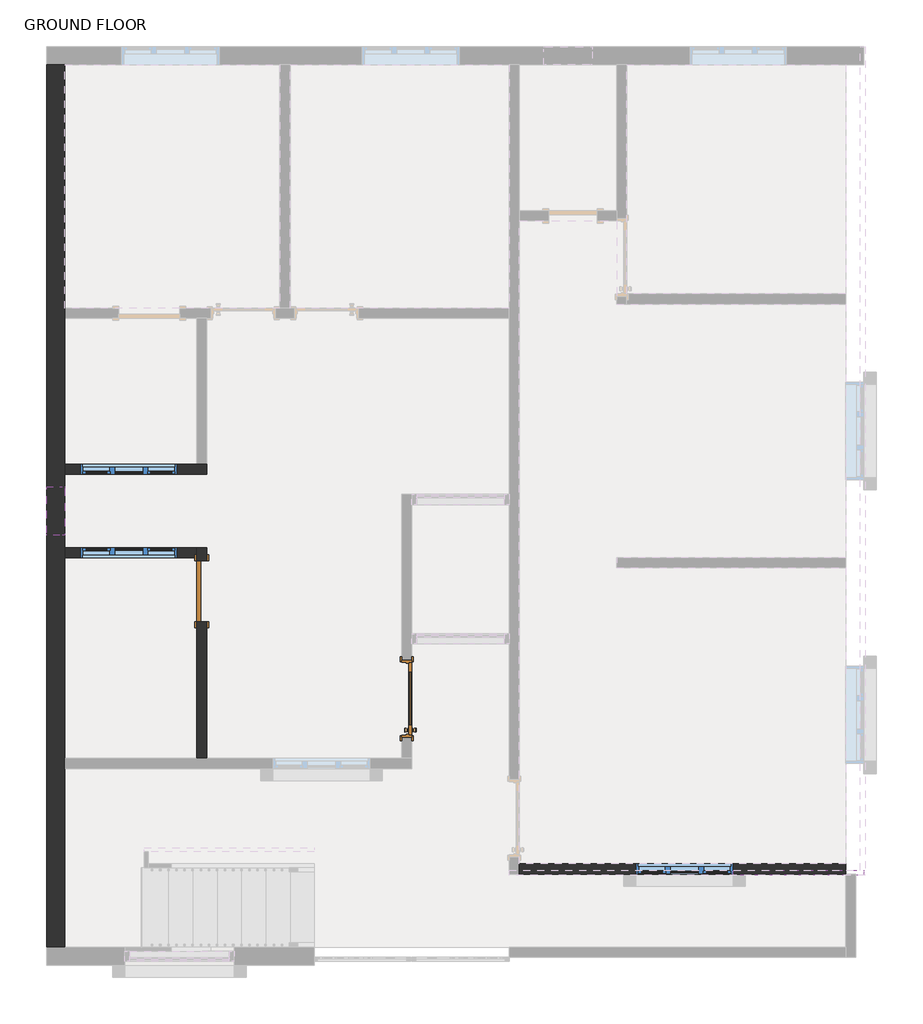
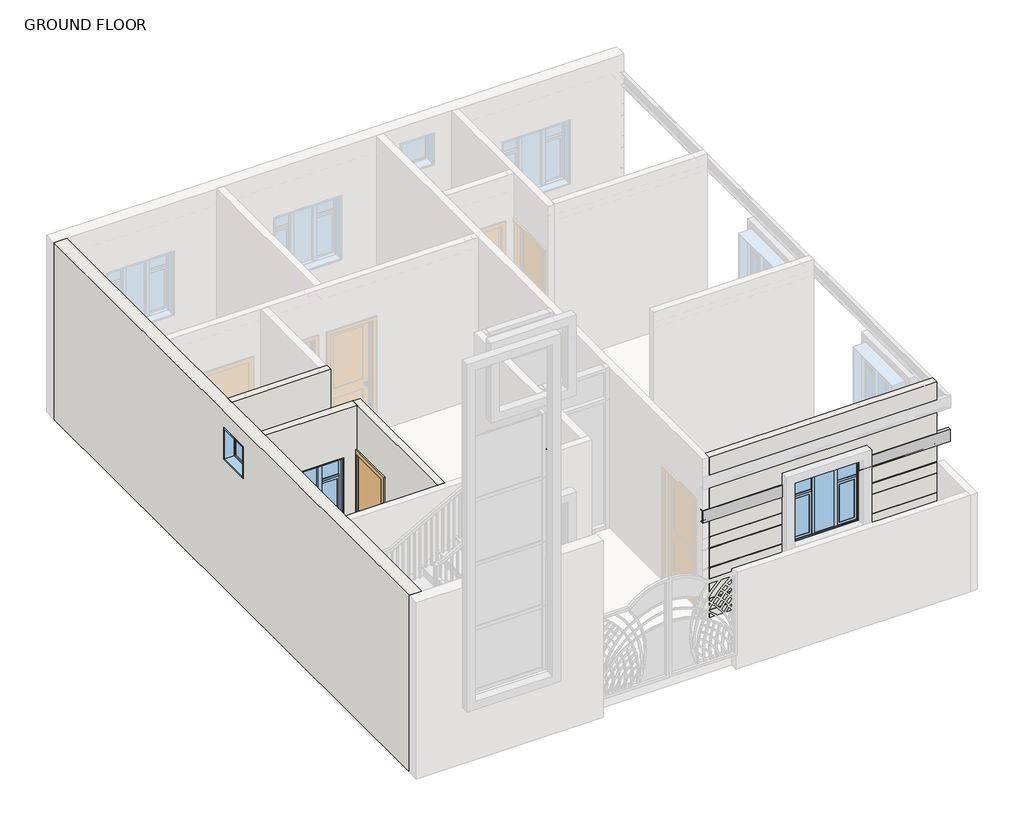
# One storey, part 2 of 7: 5 walls, 4 windows, 2 doors, 1 proxy.
"""IFC4 building model written with IfcOpenShell, lengths in millimetres."""

from ifc_helpers import new_model, si_unit, point, frame, frame_2d, origin, place, context, project, spatial, polyline, circle_curve, trimmed, segment, composite_curve, outline, extrude, faceted_brep, transform, mapped, element, save
from ifc_brep_helpers import plane_surface, cylinder_surface, revolved_surface, advanced_brep
from components import door_2e56f206, single_flush_bathroom_flush_door_4d6c7550, fixed_opening_window_2_x_2_e119d648, window_casement_triple_side_transom_window_4_x_4_9406f89d

model = new_model("IFC4")

# Units and contexts
model_context = context("Model", 3, world=origin())
ifc_project = project(units=[si_unit("LENGTHUNIT", "METRE", prefix="MILLI")], contexts=[model_context])

# Site, building, storey
site = spatial("IfcSite", under=ifc_project)
building = spatial("IfcBuilding", under=site)
storey = spatial("IfcBuildingStorey", under=building, Name="GROUND FLOOR", Elevation=304.8)

# Proxy
placement = place(None, origin())
element("IfcBuildingElementProxy", 1, Name="Reveal", ObjectType="Reveal", at=placement, inside=storey, context=model_context, shape_type="SweptSolid", body=[
    extrude(outline(composite_curve([segment(polyline([(-1857.2343863, 2374.9), (-1793.9883863, 2374.9), (-1793.9883863, 2373.5203242)]), True, "CONTINUOUS"), segment(trimmed(circle_curve(frame_2d((-1799.2334863, 2373.5203242)), 5.2451), [point((-1793.9883863, 2373.5203242))], [point((-1798.3711955, 2368.3465897))], False, "CARTESIAN"), True, "CONTINUOUS"), segment(polyline([(-1798.3711955, 2368.3465897), (-1821.9918863, 2364.4098), (-1841.2297679, 2361.20348)]), True, "CONTINUOUS"), segment(trimmed(circle_curve(frame_2d((-1839.5051863, 2350.856011)), 10.4902), [point((-1841.2297679, 2361.20348))], [point((-1849.9953863, 2350.856011))], True, "CARTESIAN"), True, "CONTINUOUS"), segment(polyline([(-1849.9953863, 2350.856011), (-1849.9953863, 2170.343989)]), True, "CONTINUOUS"), segment(trimmed(circle_curve(frame_2d((-1839.5051863, 2170.343989)), 10.4902), [point((-1849.9953863, 2170.343989))], [point((-1841.2297679, 2159.99652))], True, "CARTESIAN"), True, "CONTINUOUS"), segment(polyline([(-1841.2297679, 2159.99652), (-1821.9918863, 2156.7902), (-1798.3711955, 2152.8534103)]), True, "CONTINUOUS"), segment(trimmed(circle_curve(frame_2d((-1799.2334863, 2147.6796758)), 5.2451), [point((-1798.3711955, 2152.8534103))], [point((-1793.9883863, 2147.6796758))], False, "CARTESIAN"), True, "CONTINUOUS"), segment(polyline([(-1793.9883863, 2147.6796758), (-1793.9883863, 2146.3), (-1857.2343863, 2146.3), (-1857.2343863, 2374.9)]), True, "CONTINUOUS")], self_intersect=False)), frame((-6391.4023867, 0.0, 0.0), z_axis=(1.0, 0.0, 0.0), x_axis=(0.0, 1.0, 0.0)), (0.0, 0.0, 1.0), 1638.3),
    extrude(outline(composite_curve([segment(polyline([(-1857.2343863, 2374.9), (-1793.9883863, 2374.9), (-1793.9883863, 2373.5203242)]), True, "CONTINUOUS"), segment(trimmed(circle_curve(frame_2d((-1799.2334863, 2373.5203242)), 5.2451), [point((-1793.9883863, 2373.5203242))], [point((-1798.3711955, 2368.3465897))], False, "CARTESIAN"), True, "CONTINUOUS"), segment(polyline([(-1798.3711955, 2368.3465897), (-1821.9918863, 2364.4098), (-1841.2297679, 2361.20348)]), True, "CONTINUOUS"), segment(trimmed(circle_curve(frame_2d((-1839.5051863, 2350.856011)), 10.4902), [point((-1841.2297679, 2361.20348))], [point((-1849.9953863, 2350.856011))], True, "CARTESIAN"), True, "CONTINUOUS"), segment(polyline([(-1849.9953863, 2350.856011), (-1849.9953863, 2170.343989)]), True, "CONTINUOUS"), segment(trimmed(circle_curve(frame_2d((-1839.5051863, 2170.343989)), 10.4902), [point((-1849.9953863, 2170.343989))], [point((-1841.2297679, 2159.99652))], True, "CARTESIAN"), True, "CONTINUOUS"), segment(polyline([(-1841.2297679, 2159.99652), (-1821.9918863, 2156.7902), (-1798.3711955, 2152.8534103)]), True, "CONTINUOUS"), segment(trimmed(circle_curve(frame_2d((-1799.2334863, 2147.6796758)), 5.2451), [point((-1798.3711955, 2152.8534103))], [point((-1793.9883863, 2147.6796758))], False, "CARTESIAN"), True, "CONTINUOUS"), segment(polyline([(-1793.9883863, 2147.6796758), (-1793.9883863, 2146.3), (-1857.2343863, 2146.3), (-1857.2343863, 2374.9)]), True, "CONTINUOUS")], self_intersect=False)), frame((-9198.1023867, 0.0, 0.0), z_axis=(1.0, 0.0, 0.0), x_axis=(0.0, 1.0, 0.0)), (0.0, 0.0, 1.0), 1587.5),
])

# Doors
door_shape = door_2e56f206(model_context)
element("IfcDoor", 2, ObjectType="Door-Interior-Single-2_Panel-Wood : 36\" x 84\"", at=placement, inside=storey, context=model_context, shape_type="MappedRepresentation", body=[
    mapped(door_shape, transform((-10477.6273867, 354.7500137, 304.8), x_axis=(0.0, 1.0, 0.0), y_axis=(-1.0, 0.0, 0.0), z_axis=(0.0, 0.0, 1.0))),
])
single_flush_bathroom_flush_door_shape = single_flush_bathroom_flush_door_4d6c7550(model_context)
element("IfcDoor", 3, ObjectType="Single-Flush : BATHROOM FLUSH DOOR", at=placement, inside=storey, context=model_context, shape_type="MappedRepresentation", body=[
    mapped(single_flush_bathroom_flush_door_shape, transform((-13046.2023867, 1700.5265627, 304.8), x_axis=(0.0, 1.0, 0.0), y_axis=(-1.0, 0.0, 0.0), z_axis=(0.0, 0.0, 1.0))),
])

# Walls
element("IfcWall", 4, at=placement, inside=storey, context=model_context, shape_type="Brep", body=[
    faceted_brep([(-14760.7023867, -2756.7499863, 0.0), (-14760.7023867, 8292.2500137, 0.0), (-14760.7023867, 8292.2500137, 3352.8), (-14760.7023867, 5244.2500137, 3352.8), (-14760.7023867, 5117.2500137, 3352.8), (-14760.7023867, 3288.4500137, 3352.8), (-14760.7023867, 3161.4500137, 3352.8), (-14760.7023867, 2246.6265627, 3352.8), (-14760.7023867, 2119.6265627, 3352.8), (-14760.7023867, -394.5499863, 3352.8), (-14760.7023867, -521.5499863, 3352.8), (-14760.7023867, -2756.7499863, 3352.8), (-14760.7023867, 2399.2382882, 2438.4), (-14760.7023867, 2399.2382882, 3048.0), (-14760.7023867, 3008.8382882, 3048.0), (-14760.7023867, 3008.8382882, 2438.4), (-14989.3023867, 8292.2500137, 0.0), (-14989.3023867, -2756.7499863, 0.0), (-14989.3023867, -2756.7499863, 3352.8), (-14989.3023867, 8292.2500137, 3352.8), (-14989.3023867, 2399.2382882, 3048.0), (-14989.3023867, 2399.2382882, 2438.4), (-14989.3023867, 3008.8382882, 2438.4), (-14989.3023867, 3008.8382882, 3048.0)], [[[0, 1, 2, 3, 4, 5, 6, 7, 8, 9, 10, 11], [12, 13, 14, 15]], [[16, 17, 18, 19], [20, 21, 22, 23]], [[1, 0, 17, 16]], [[11, 10, 9, 8, 7, 6, 5, 4, 3, 2, 19, 18]], [[0, 11, 18, 17]], [[2, 1, 16, 19]], [[20, 13, 12, 21]], [[21, 12, 15, 22]], [[22, 15, 14, 23]], [[13, 20, 23, 14]]]),
])
element("IfcWall", 5, ObjectType="INNER WALL 5\"", at=placement, inside=storey, context=model_context, shape_type="AdvancedBrep", body=[
    advanced_brep(
    [(-9071.1023867, -1842.3499863, 0.0), (-4981.7023867, -1842.3499863, 0.0), (-4981.7023867, -1842.3499863, 444.5), (-9071.1023867, -1842.3499863, 444.5), (-9071.1023867, -1842.3499863, 304.8), (-4981.7023867, -1842.3499863, 3352.8), (-9071.1023867, -1842.3499863, 3352.8), (-9071.1023867, -1842.3499863, 3009.9), (-4981.7023867, -1842.3499863, 3009.9), (-6391.4023867, -1842.3499863, 1219.2), (-7610.6023867, -1842.3499863, 1219.2), (-7610.6023867, -1842.3499863, 1243.35311), (-9071.1023867, -1842.3499863, 1243.35311), (-9071.1023867, -1842.3499863, 1042.64689), (-4981.7023867, -1842.3499863, 1042.64689), (-4981.7023867, -1842.3499863, 1243.35311), (-6391.4023867, -1842.3499863, 1243.35311), (-7610.6023867, -1842.3499863, 2438.4), (-6391.4023867, -1842.3499863, 2438.4), (-6391.4023867, -1842.3499863, 2374.9), (-4981.7023867, -1842.3499863, 2374.9), (-4981.7023867, -1842.3499863, 2781.3), (-9071.1023867, -1842.3499863, 2781.3), (-9071.1023867, -1842.3499863, 2374.9), (-7610.6023867, -1842.3499863, 2374.9), (-4981.7023867, -1842.3499863, 2795.24689), (-4981.7023867, -1842.3499863, 2995.95311), (-9071.1023867, -1842.3499863, 2995.95311), (-9071.1023867, -1842.3499863, 2795.24689), (-9071.1023867, -1842.3499863, 673.1), (-4981.7023867, -1842.3499863, 673.1), (-4981.7023867, -1842.3499863, 1028.7), (-9071.1023867, -1842.3499863, 1028.7), (-4981.7023867, -1842.3499863, 659.15311), (-9071.1023867, -1842.3499863, 659.15311), (-9071.1023867, -1842.3499863, 458.44689), (-4981.7023867, -1842.3499863, 458.44689), (-9071.1023867, -1842.3499863, 1257.3), (-7610.6023867, -1842.3499863, 1257.3), (-7610.6023867, -1842.3499863, 1612.9), (-9071.1023867, -1842.3499863, 1612.9), (-6391.4023867, -1842.3499863, 1257.3), (-4981.7023867, -1842.3499863, 1257.3), (-4981.7023867, -1842.3499863, 1612.9), (-6391.4023867, -1842.3499863, 1612.9), (-6391.4023867, -1842.3499863, 1841.5), (-4981.7023867, -1842.3499863, 1841.5), (-4981.7023867, -1842.3499863, 2146.3), (-6391.4023867, -1842.3499863, 2146.3), (-4981.7023867, -1842.3499863, 1827.55311), (-6391.4023867, -1842.3499863, 1827.55311), (-6391.4023867, -1842.3499863, 1626.84689), (-4981.7023867, -1842.3499863, 1626.84689), (-9071.1023867, -1842.3499863, 1841.5), (-7610.6023867, -1842.3499863, 1841.5), (-7610.6023867, -1842.3499863, 2146.3), (-9071.1023867, -1842.3499863, 2146.3), (-7610.6023867, -1842.3499863, 1827.55311), (-9071.1023867, -1842.3499863, 1827.55311), (-9071.1023867, -1842.3499863, 1626.84689), (-7610.6023867, -1842.3499863, 1626.84689), (-6391.4023867, -1842.3499863, 2360.95311), (-6391.4023867, -1842.3499863, 2160.24689), (-4981.7023867, -1842.3499863, 2160.24689), (-4981.7023867, -1842.3499863, 2360.95311), (-9071.1023867, -1842.3499863, 2360.95311), (-9071.1023867, -1842.3499863, 2160.24689), (-7610.6023867, -1842.3499863, 2160.24689), (-7610.6023867, -1842.3499863, 2360.95311), (-4981.7023867, -1715.3499863, 0.0), (-9071.1023867, -1715.3499863, 0.0), (-9071.1023867, -1715.3499863, 3352.8), (-4981.7023867, -1715.3499863, 3352.8), (-7610.6023867, -1715.3499863, 2438.4), (-7610.6023867, -1715.3499863, 1219.2), (-6391.4023867, -1715.3499863, 1219.2), (-6391.4023867, -1715.3499863, 2438.4), (-9071.1023867, -1793.9883863, 444.5), (-9071.1023867, -1793.9883863, 445.8796758), (-9071.1023867, -1798.3711955, 451.0534103), (-9071.1023867, -1841.2297679, 458.19652), (-9071.1023867, -1841.2297679, 659.40348), (-9071.1023867, -1798.3711955, 666.5465897), (-9071.1023867, -1793.9883863, 671.7203242), (-9071.1023867, -1793.9883863, 673.1), (-9071.1023867, -1793.9883863, 1028.7), (-9071.1023867, -1793.9883863, 1030.0796758), (-9071.1023867, -1798.3711955, 1035.2534103), (-9071.1023867, -1841.2297679, 1042.39652), (-9071.1023867, -1841.2297679, 1243.60348), (-9071.1023867, -1798.3711955, 1250.7465897), (-9071.1023867, -1793.9883863, 1255.9203242), (-9071.1023867, -1793.9883863, 1257.3), (-9071.1023867, -1793.9883863, 1612.9), (-9071.1023867, -1793.9883863, 1614.2796758), (-9071.1023867, -1798.3711955, 1619.4534103), (-9071.1023867, -1841.2297679, 1626.59652), (-9071.1023867, -1841.2297679, 1827.80348), (-9071.1023867, -1798.3711955, 1834.9465897), (-9071.1023867, -1793.9883863, 1840.1203242), (-9071.1023867, -1793.9883863, 1841.5), (-9071.1023867, -1793.9883863, 2146.3), (-9071.1023867, -1793.9883863, 2147.6796758), (-9071.1023867, -1798.3711955, 2152.8534103), (-9071.1023867, -1841.2297679, 2159.99652), (-9071.1023867, -1841.2297679, 2361.20348), (-9071.1023867, -1798.3711955, 2368.3465897), (-9071.1023867, -1793.9883863, 2373.5203242), (-9071.1023867, -1793.9883863, 2374.9), (-9071.1023867, -1793.9883863, 2781.3), (-9071.1023867, -1793.9883863, 2782.6796758), (-9071.1023867, -1798.3711955, 2787.8534103), (-9071.1023867, -1841.2297679, 2794.99652), (-9071.1023867, -1841.2297679, 2996.20348), (-9071.1023867, -1798.3711955, 3003.3465897), (-9071.1023867, -1793.9883863, 3008.5203242), (-9071.1023867, -1793.9883863, 3009.9), (-7610.6023867, -1793.9883863, 2374.9), (-7610.6023867, -1793.9883863, 2373.5203242), (-7610.6023867, -1798.3711955, 2368.3465897), (-7610.6023867, -1841.2297679, 2361.20348), (-7610.6023867, -1841.2297679, 2159.99652), (-7610.6023867, -1798.3711955, 2152.8534103), (-7610.6023867, -1793.9883863, 2147.6796758), (-7610.6023867, -1793.9883863, 2146.3), (-7610.6023867, -1793.9883863, 1841.5), (-7610.6023867, -1793.9883863, 1840.1203242), (-7610.6023867, -1798.3711955, 1834.9465897), (-7610.6023867, -1841.2297679, 1827.80348), (-7610.6023867, -1841.2297679, 1626.59652), (-7610.6023867, -1798.3711955, 1619.4534103), (-7610.6023867, -1793.9883863, 1614.2796758), (-7610.6023867, -1793.9883863, 1612.9), (-7610.6023867, -1793.9883863, 1257.3), (-7610.6023867, -1793.9883863, 1255.9203242), (-7610.6023867, -1798.3711955, 1250.7465897), (-7610.6023867, -1841.2297679, 1243.60348), (-6391.4023867, -1841.2297679, 1243.60348), (-6391.4023867, -1798.3711955, 1250.7465897), (-6391.4023867, -1793.9883863, 1255.9203242), (-6391.4023867, -1793.9883863, 1257.3), (-6391.4023867, -1793.9883863, 1612.9), (-6391.4023867, -1793.9883863, 1614.2796758), (-6391.4023867, -1798.3711955, 1619.4534103), (-6391.4023867, -1841.2297679, 1626.59652), (-6391.4023867, -1841.2297679, 1827.80348), (-6391.4023867, -1798.3711955, 1834.9465897), (-6391.4023867, -1793.9883863, 1840.1203242), (-6391.4023867, -1793.9883863, 1841.5), (-6391.4023867, -1793.9883863, 2146.3), (-6391.4023867, -1793.9883863, 2147.6796758), (-6391.4023867, -1798.3711955, 2152.8534103), (-6391.4023867, -1841.2297679, 2159.99652), (-6391.4023867, -1841.2297679, 2361.20348), (-6391.4023867, -1798.3711955, 2368.3465897), (-6391.4023867, -1793.9883863, 2373.5203242), (-6391.4023867, -1793.9883863, 2374.9), (-4981.7023867, -1793.9883863, 3009.9), (-4981.7023867, -1793.9883863, 3008.5203242), (-4981.7023867, -1798.3711955, 3003.3465897), (-4981.7023867, -1841.2297679, 2996.20348), (-4981.7023867, -1841.2297679, 2794.99652), (-4981.7023867, -1798.3711955, 2787.8534103), (-4981.7023867, -1793.9883863, 2782.6796758), (-4981.7023867, -1793.9883863, 2781.3), (-4981.7023867, -1793.9883863, 2374.9), (-4981.7023867, -1793.9883863, 2373.5203242), (-4981.7023867, -1798.3711955, 2368.3465897), (-4981.7023867, -1841.2297679, 2361.20348), (-4981.7023867, -1841.2297679, 2159.99652), (-4981.7023867, -1798.3711955, 2152.8534103), (-4981.7023867, -1793.9883863, 2147.6796758), (-4981.7023867, -1793.9883863, 2146.3), (-4981.7023867, -1793.9883863, 1841.5), (-4981.7023867, -1793.9883863, 1840.1203242), (-4981.7023867, -1798.3711955, 1834.9465897), (-4981.7023867, -1841.2297679, 1827.80348), (-4981.7023867, -1841.2297679, 1626.59652), (-4981.7023867, -1798.3711955, 1619.4534103), (-4981.7023867, -1793.9883863, 1614.2796758), (-4981.7023867, -1793.9883863, 1612.9), (-4981.7023867, -1793.9883863, 1257.3), (-4981.7023867, -1793.9883863, 1255.9203242), (-4981.7023867, -1798.3711955, 1250.7465897), (-4981.7023867, -1841.2297679, 1243.60348), (-4981.7023867, -1841.2297679, 1042.39652), (-4981.7023867, -1798.3711955, 1035.2534103), (-4981.7023867, -1793.9883863, 1030.0796758), (-4981.7023867, -1793.9883863, 1028.7), (-4981.7023867, -1793.9883863, 673.1), (-4981.7023867, -1793.9883863, 671.7203242), (-4981.7023867, -1798.3711955, 666.5465897), (-4981.7023867, -1841.2297679, 659.40348), (-4981.7023867, -1841.2297679, 458.19652), (-4981.7023867, -1798.3711955, 451.0534103), (-4981.7023867, -1793.9883863, 445.8796758), (-4981.7023867, -1793.9883863, 444.5)],
    [
        (0, 1),
        (1, 2),
        (2, 3),
        (3, 4),
        (4, 0),
        (5, 6),
        (6, 7),
        (7, 8),
        (8, 5),
        (9, 10),
        (10, 11),
        (11, 12),
        (12, 13),
        (13, 14),
        (14, 15),
        (15, 16),
        (16, 9),
        (17, 18),
        (18, 19),
        (19, 20),
        (20, 21),
        (21, 22),
        (22, 23),
        (23, 24),
        (24, 17),
        (25, 26),
        (26, 27),
        (27, 28),
        (28, 25),
        (29, 30),
        (30, 31),
        (31, 32),
        (32, 29),
        (33, 34),
        (34, 35),
        (35, 36),
        (36, 33),
        (37, 38),
        (38, 39),
        (39, 40),
        (40, 37),
        (41, 42),
        (42, 43),
        (43, 44),
        (44, 41),
        (45, 46),
        (46, 47),
        (47, 48),
        (48, 45),
        (49, 50),
        (50, 51),
        (51, 52),
        (52, 49),
        (53, 54),
        (54, 55),
        (55, 56),
        (56, 53),
        (57, 58),
        (58, 59),
        (59, 60),
        (60, 57),
        (61, 62),
        (62, 63),
        (63, 64),
        (64, 61),
        (65, 66),
        (66, 67),
        (67, 68),
        (68, 65),
        (69, 70),
        (70, 71),
        (71, 72),
        (72, 69),
        (73, 74),
        (74, 75),
        (75, 76),
        (76, 73),
        (0, 70),
        (69, 1),
        (5, 72),
        (71, 6),
        (3, 77),
        (77, 78),
        (78, 79, circle_curve(frame((-9071.1023867, -1799.2334863, 445.8796758), z_axis=(1.0, 0.0, 0.0), x_axis=(0.0, 1.0, 0.0)), 5.2451)),
        (79, 80),
        (80, 35, circle_curve(frame((-9071.1023867, -1839.5051863, 468.543989), z_axis=(-1.0, 0.0, 0.0), x_axis=(0.0, 1.0, 0.0)), 10.4902)),
        (34, 81, circle_curve(frame((-9071.1023867, -1839.5051863, 649.056011), z_axis=(-1.0, 0.0, 0.0), x_axis=(0.0, 1.0, 0.0)), 10.4902)),
        (81, 82),
        (82, 83, circle_curve(frame((-9071.1023867, -1799.2334863, 671.7203242), z_axis=(1.0, 0.0, 0.0), x_axis=(0.0, 1.0, 0.0)), 5.2451)),
        (83, 84),
        (84, 29),
        (32, 85),
        (85, 86),
        (86, 87, circle_curve(frame((-9071.1023867, -1799.2334863, 1030.0796758), z_axis=(1.0, 0.0, 0.0), x_axis=(0.0, 1.0, 0.0)), 5.2451)),
        (87, 88),
        (88, 13, circle_curve(frame((-9071.1023867, -1839.5051863, 1052.743989), z_axis=(-1.0, 0.0, 0.0), x_axis=(0.0, 1.0, 0.0)), 10.4902)),
        (12, 89, circle_curve(frame((-9071.1023867, -1839.5051863, 1233.256011), z_axis=(-1.0, 0.0, 0.0), x_axis=(0.0, 1.0, 0.0)), 10.4902)),
        (89, 90),
        (90, 91, circle_curve(frame((-9071.1023867, -1799.2334863, 1255.9203242), z_axis=(1.0, 0.0, 0.0), x_axis=(0.0, 1.0, 0.0)), 5.2451)),
        (91, 92),
        (92, 37),
        (40, 93),
        (93, 94),
        (94, 95, circle_curve(frame((-9071.1023867, -1799.2334863, 1614.2796758), z_axis=(1.0, 0.0, 0.0), x_axis=(0.0, 1.0, 0.0)), 5.2451)),
        (95, 96),
        (96, 59, circle_curve(frame((-9071.1023867, -1839.5051863, 1636.943989), z_axis=(-1.0, 0.0, 0.0), x_axis=(0.0, 1.0, 0.0)), 10.4902)),
        (58, 97, circle_curve(frame((-9071.1023867, -1839.5051863, 1817.456011), z_axis=(-1.0, 0.0, 0.0), x_axis=(0.0, 1.0, 0.0)), 10.4902)),
        (97, 98),
        (98, 99, circle_curve(frame((-9071.1023867, -1799.2334863, 1840.1203242), z_axis=(1.0, 0.0, 0.0), x_axis=(0.0, 1.0, 0.0)), 5.2451)),
        (99, 100),
        (100, 53),
        (56, 101),
        (101, 102),
        (102, 103, circle_curve(frame((-9071.1023867, -1799.2334863, 2147.6796758), z_axis=(1.0, 0.0, 0.0), x_axis=(0.0, 1.0, 0.0)), 5.2451)),
        (103, 104),
        (104, 66, circle_curve(frame((-9071.1023867, -1839.5051863, 2170.343989), z_axis=(-1.0, 0.0, 0.0), x_axis=(0.0, 1.0, 0.0)), 10.4902)),
        (65, 105, circle_curve(frame((-9071.1023867, -1839.5051863, 2350.856011), z_axis=(-1.0, 0.0, 0.0), x_axis=(0.0, 1.0, 0.0)), 10.4902)),
        (105, 106),
        (106, 107, circle_curve(frame((-9071.1023867, -1799.2334863, 2373.5203242), z_axis=(1.0, 0.0, 0.0), x_axis=(0.0, 1.0, 0.0)), 5.2451)),
        (107, 108),
        (108, 23),
        (22, 109),
        (109, 110),
        (110, 111, circle_curve(frame((-9071.1023867, -1799.2334863, 2782.6796758), z_axis=(1.0, 0.0, 0.0), x_axis=(0.0, 1.0, 0.0)), 5.2451)),
        (111, 112),
        (112, 28, circle_curve(frame((-9071.1023867, -1839.5051863, 2805.343989), z_axis=(-1.0, 0.0, 0.0), x_axis=(0.0, 1.0, 0.0)), 10.4902)),
        (27, 113, circle_curve(frame((-9071.1023867, -1839.5051863, 2985.856011), z_axis=(-1.0, 0.0, 0.0), x_axis=(0.0, 1.0, 0.0)), 10.4902)),
        (113, 114),
        (114, 115, circle_curve(frame((-9071.1023867, -1799.2334863, 3008.5203242), z_axis=(1.0, 0.0, 0.0), x_axis=(0.0, 1.0, 0.0)), 5.2451)),
        (115, 116),
        (116, 7),
        (73, 17),
        (24, 117),
        (117, 118),
        (118, 119, circle_curve(frame((-7610.6023867, -1799.2334863, 2373.5203242), z_axis=(-1.0, 0.0, 0.0), x_axis=(0.0, 1.0, 0.0)), 5.2451)),
        (119, 120),
        (120, 68, circle_curve(frame((-7610.6023867, -1839.5051863, 2350.856011), z_axis=(1.0, 0.0, 0.0), x_axis=(0.0, 1.0, 0.0)), 10.4902)),
        (67, 121, circle_curve(frame((-7610.6023867, -1839.5051863, 2170.343989), z_axis=(1.0, 0.0, 0.0), x_axis=(0.0, 1.0, 0.0)), 10.4902)),
        (121, 122),
        (122, 123, circle_curve(frame((-7610.6023867, -1799.2334863, 2147.6796758), z_axis=(-1.0, 0.0, 0.0), x_axis=(0.0, 1.0, 0.0)), 5.2451)),
        (123, 124),
        (124, 55),
        (54, 125),
        (125, 126),
        (126, 127, circle_curve(frame((-7610.6023867, -1799.2334863, 1840.1203242), z_axis=(-1.0, 0.0, 0.0), x_axis=(0.0, 1.0, 0.0)), 5.2451)),
        (127, 128),
        (128, 57, circle_curve(frame((-7610.6023867, -1839.5051863, 1817.456011), z_axis=(1.0, 0.0, 0.0), x_axis=(0.0, 1.0, 0.0)), 10.4902)),
        (60, 129, circle_curve(frame((-7610.6023867, -1839.5051863, 1636.943989), z_axis=(1.0, 0.0, 0.0), x_axis=(0.0, 1.0, 0.0)), 10.4902)),
        (129, 130),
        (130, 131, circle_curve(frame((-7610.6023867, -1799.2334863, 1614.2796758), z_axis=(-1.0, 0.0, 0.0), x_axis=(0.0, 1.0, 0.0)), 5.2451)),
        (131, 132),
        (132, 39),
        (38, 133),
        (133, 134),
        (134, 135, circle_curve(frame((-7610.6023867, -1799.2334863, 1255.9203242), z_axis=(-1.0, 0.0, 0.0), x_axis=(0.0, 1.0, 0.0)), 5.2451)),
        (135, 136),
        (136, 11, circle_curve(frame((-7610.6023867, -1839.5051863, 1233.256011), z_axis=(1.0, 0.0, 0.0), x_axis=(0.0, 1.0, 0.0)), 10.4902)),
        (10, 74),
        (9, 75),
        (16, 137, circle_curve(frame((-6391.4023867, -1839.5051863, 1233.256011), z_axis=(-1.0, 0.0, 0.0), x_axis=(0.0, 1.0, 0.0)), 10.4902)),
        (137, 138),
        (138, 139, circle_curve(frame((-6391.4023867, -1799.2334863, 1255.9203242), z_axis=(1.0, 0.0, 0.0), x_axis=(0.0, 1.0, 0.0)), 5.2451)),
        (139, 140),
        (140, 41),
        (44, 141),
        (141, 142),
        (142, 143, circle_curve(frame((-6391.4023867, -1799.2334863, 1614.2796758), z_axis=(1.0, 0.0, 0.0), x_axis=(0.0, 1.0, 0.0)), 5.2451)),
        (143, 144),
        (144, 51, circle_curve(frame((-6391.4023867, -1839.5051863, 1636.943989), z_axis=(-1.0, 0.0, 0.0), x_axis=(0.0, 1.0, 0.0)), 10.4902)),
        (50, 145, circle_curve(frame((-6391.4023867, -1839.5051863, 1817.456011), z_axis=(-1.0, 0.0, 0.0), x_axis=(0.0, 1.0, 0.0)), 10.4902)),
        (145, 146),
        (146, 147, circle_curve(frame((-6391.4023867, -1799.2334863, 1840.1203242), z_axis=(1.0, 0.0, 0.0), x_axis=(0.0, 1.0, 0.0)), 5.2451)),
        (147, 148),
        (148, 45),
        (48, 149),
        (149, 150),
        (150, 151, circle_curve(frame((-6391.4023867, -1799.2334863, 2147.6796758), z_axis=(1.0, 0.0, 0.0), x_axis=(0.0, 1.0, 0.0)), 5.2451)),
        (151, 152),
        (152, 62, circle_curve(frame((-6391.4023867, -1839.5051863, 2170.343989), z_axis=(-1.0, 0.0, 0.0), x_axis=(0.0, 1.0, 0.0)), 10.4902)),
        (61, 153, circle_curve(frame((-6391.4023867, -1839.5051863, 2350.856011), z_axis=(-1.0, 0.0, 0.0), x_axis=(0.0, 1.0, 0.0)), 10.4902)),
        (153, 154),
        (154, 155, circle_curve(frame((-6391.4023867, -1799.2334863, 2373.5203242), z_axis=(1.0, 0.0, 0.0), x_axis=(0.0, 1.0, 0.0)), 5.2451)),
        (155, 156),
        (156, 19),
        (18, 76),
        (8, 157),
        (157, 158),
        (158, 159, circle_curve(frame((-4981.7023867, -1799.2334863, 3008.5203242), z_axis=(-1.0, 0.0, 0.0), x_axis=(0.0, 1.0, 0.0)), 5.2451)),
        (159, 160),
        (160, 26, circle_curve(frame((-4981.7023867, -1839.5051863, 2985.856011), z_axis=(1.0, 0.0, 0.0), x_axis=(0.0, 1.0, 0.0)), 10.4902)),
        (25, 161, circle_curve(frame((-4981.7023867, -1839.5051863, 2805.343989), z_axis=(1.0, 0.0, 0.0), x_axis=(0.0, 1.0, 0.0)), 10.4902)),
        (161, 162),
        (162, 163, circle_curve(frame((-4981.7023867, -1799.2334863, 2782.6796758), z_axis=(-1.0, 0.0, 0.0), x_axis=(0.0, 1.0, 0.0)), 5.2451)),
        (163, 164),
        (164, 21),
        (20, 165),
        (165, 166),
        (166, 167, circle_curve(frame((-4981.7023867, -1799.2334863, 2373.5203242), z_axis=(-1.0, 0.0, 0.0), x_axis=(0.0, 1.0, 0.0)), 5.2451)),
        (167, 168),
        (168, 64, circle_curve(frame((-4981.7023867, -1839.5051863, 2350.856011), z_axis=(1.0, 0.0, 0.0), x_axis=(0.0, 1.0, 0.0)), 10.4902)),
        (63, 169, circle_curve(frame((-4981.7023867, -1839.5051863, 2170.343989), z_axis=(1.0, 0.0, 0.0), x_axis=(0.0, 1.0, 0.0)), 10.4902)),
        (169, 170),
        (170, 171, circle_curve(frame((-4981.7023867, -1799.2334863, 2147.6796758), z_axis=(-1.0, 0.0, 0.0), x_axis=(0.0, 1.0, 0.0)), 5.2451)),
        (171, 172),
        (172, 47),
        (46, 173),
        (173, 174),
        (174, 175, circle_curve(frame((-4981.7023867, -1799.2334863, 1840.1203242), z_axis=(-1.0, 0.0, 0.0), x_axis=(0.0, 1.0, 0.0)), 5.2451)),
        (175, 176),
        (176, 49, circle_curve(frame((-4981.7023867, -1839.5051863, 1817.456011), z_axis=(1.0, 0.0, 0.0), x_axis=(0.0, 1.0, 0.0)), 10.4902)),
        (52, 177, circle_curve(frame((-4981.7023867, -1839.5051863, 1636.943989), z_axis=(1.0, 0.0, 0.0), x_axis=(0.0, 1.0, 0.0)), 10.4902)),
        (177, 178),
        (178, 179, circle_curve(frame((-4981.7023867, -1799.2334863, 1614.2796758), z_axis=(-1.0, 0.0, 0.0), x_axis=(0.0, 1.0, 0.0)), 5.2451)),
        (179, 180),
        (180, 43),
        (42, 181),
        (181, 182),
        (182, 183, circle_curve(frame((-4981.7023867, -1799.2334863, 1255.9203242), z_axis=(-1.0, 0.0, 0.0), x_axis=(0.0, 1.0, 0.0)), 5.2451)),
        (183, 184),
        (184, 15, circle_curve(frame((-4981.7023867, -1839.5051863, 1233.256011), z_axis=(1.0, 0.0, 0.0), x_axis=(0.0, 1.0, 0.0)), 10.4902)),
        (14, 185, circle_curve(frame((-4981.7023867, -1839.5051863, 1052.743989), z_axis=(1.0, 0.0, 0.0), x_axis=(0.0, 1.0, 0.0)), 10.4902)),
        (185, 186),
        (186, 187, circle_curve(frame((-4981.7023867, -1799.2334863, 1030.0796758), z_axis=(-1.0, 0.0, 0.0), x_axis=(0.0, 1.0, 0.0)), 5.2451)),
        (187, 188),
        (188, 31),
        (30, 189),
        (189, 190),
        (190, 191, circle_curve(frame((-4981.7023867, -1799.2334863, 671.7203242), z_axis=(-1.0, 0.0, 0.0), x_axis=(0.0, 1.0, 0.0)), 5.2451)),
        (191, 192),
        (192, 33, circle_curve(frame((-4981.7023867, -1839.5051863, 649.056011), z_axis=(1.0, 0.0, 0.0), x_axis=(0.0, 1.0, 0.0)), 10.4902)),
        (36, 193, circle_curve(frame((-4981.7023867, -1839.5051863, 468.543989), z_axis=(1.0, 0.0, 0.0), x_axis=(0.0, 1.0, 0.0)), 10.4902)),
        (193, 194),
        (194, 195, circle_curve(frame((-4981.7023867, -1799.2334863, 445.8796758), z_axis=(-1.0, 0.0, 0.0), x_axis=(0.0, 1.0, 0.0)), 5.2451)),
        (195, 196),
        (196, 2),
        (116, 157),
        (115, 158),
        (114, 159),
        (113, 160),
        (112, 161),
        (111, 162),
        (110, 163),
        (109, 164),
        (84, 189),
        (83, 190),
        (82, 191),
        (81, 192),
        (80, 193),
        (79, 194),
        (78, 195),
        (77, 196),
        (92, 133),
        (140, 181),
        (91, 134),
        (139, 182),
        (90, 135),
        (138, 183),
        (89, 136),
        (137, 184),
        (88, 185),
        (87, 186),
        (86, 187),
        (85, 188),
        (148, 173),
        (147, 174),
        (146, 175),
        (145, 176),
        (144, 177),
        (143, 178),
        (142, 179),
        (141, 180),
        (100, 125),
        (99, 126),
        (98, 127),
        (97, 128),
        (96, 129),
        (95, 130),
        (94, 131),
        (93, 132),
        (156, 165),
        (155, 166),
        (154, 167),
        (153, 168),
        (152, 169),
        (151, 170),
        (150, 171),
        (149, 172),
        (108, 117),
        (107, 118),
        (106, 119),
        (105, 120),
        (104, 121),
        (103, 122),
        (102, 123),
        (101, 124),
    ],
    [
        plane_surface(frame((-9198.1023867, -1842.3499863, 0.0), z_axis=(0.0, -1.0, 0.0), x_axis=(1.0, 0.0, 0.0))),
        plane_surface(frame((-9198.1023867, -1715.3499863, 0.0), z_axis=(0.0, 1.0, 0.0), x_axis=(-1.0, 0.0, 0.0))),
        plane_surface(frame((-9134.6023867, -1842.3499863, 0.0), z_axis=(0.0, 0.0, -1.0), x_axis=(0.0, 1.0, 0.0))),
        plane_surface(frame((-4867.4023867, -1842.3499863, 3352.8), z_axis=(0.0, 0.0, 1.0), x_axis=(0.0, 1.0, 0.0))),
        plane_surface(frame((-9071.1023867, 8292.2500137, 304.8), z_axis=(-1.0, 0.0, 0.0), x_axis=(0.0, 1.0, 0.0))),
        plane_surface(frame((-7610.6023867, -1715.3499863, 2438.4), z_axis=(1.0, 0.0, 0.0), x_axis=(0.0, -1.0, 0.0))),
        plane_surface(frame((-7610.6023867, -1715.3499863, 1219.2), z_axis=(0.0, 0.0, 1.0), x_axis=(0.0, -1.0, 0.0))),
        plane_surface(frame((-6391.4023867, -1715.3499863, 1219.2), z_axis=(-1.0, 0.0, 0.0), x_axis=(0.0, -1.0, 0.0))),
        plane_surface(frame((-6391.4023867, -1715.3499863, 2438.4), z_axis=(0.0, 0.0, -1.0), x_axis=(0.0, -1.0, 0.0))),
        plane_surface(frame((-4981.7023867, 8520.8500137, 0.0), z_axis=(1.0, 0.0, 0.0), x_axis=(0.0, -1.0, 0.0))),
        plane_surface(frame((-9198.1023867, -1857.2343863, 3009.9), z_axis=(0.0, 0.0, -1.0), x_axis=(1.0, 0.0, 0.0))),
        plane_surface(frame((-9198.1023867, -1793.9883863, 3009.9), z_axis=(0.0, -1.0, 0.0), x_axis=(1.0, 0.0, 0.0))),
        revolved_surface(polyline([(-9071.1023867, -1793.9883863, 3008.5203242), (-4981.7023867, -1793.9883863, 3008.5203242)]), (-9198.1023867, -1799.2334863, 3008.5203242), (-1.0, 0.0, 0.0)),
        plane_surface(frame((-9198.1023867, -1821.9918863, 2999.4098), z_axis=(0.0, -0.16439930721687146, 0.9863938705135048), x_axis=(1.0, 0.0, 0.0))),
        cylinder_surface(frame((-9198.1023867, -1839.5051863, 2985.856011), z_axis=(1.0, 0.0, 0.0), x_axis=(0.0, 1.0, 0.0)), 10.4902),
        cylinder_surface(frame((-9198.1023867, -1839.5051863, 2805.343989), z_axis=(1.0, 0.0, 0.0), x_axis=(0.0, 1.0, 0.0)), 10.4902),
        plane_surface(frame((-9198.1023867, -1821.9918863, 2791.7902), z_axis=(0.0, -0.16439930721687793, -0.9863938705135037), x_axis=(1.0, 0.0, 0.0))),
        revolved_surface(polyline([(-9071.1023867, -1793.9883863, 2782.6796758), (-4981.7023867, -1793.9883863, 2782.6796758)]), (-9198.1023867, -1799.2334863, 2782.6796758), (-1.0, 0.0, 0.0)),
        plane_surface(frame((-9198.1023867, -1793.9883863, 2782.6796758), z_axis=(0.0, -1.0, 0.0), x_axis=(1.0, 0.0, 0.0))),
        plane_surface(frame((-9198.1023867, -1793.9883863, 2781.3), z_axis=(0.0, 0.0, 1.0), x_axis=(1.0, 0.0, 0.0))),
        plane_surface(frame((-9198.1023867, -1857.2343863, 673.1), z_axis=(0.0, 0.0, -1.0), x_axis=(1.0, 0.0, 0.0))),
        plane_surface(frame((-9198.1023867, -1793.9883863, 673.1), z_axis=(0.0, -1.0, 0.0), x_axis=(1.0, 0.0, 0.0))),
        revolved_surface(polyline([(-9071.1023867, -1793.9883863, 671.7203242), (-4981.7023867, -1793.9883863, 671.7203242)]), (-9198.1023867, -1799.2334863, 671.7203242), (-1.0, 0.0, 0.0)),
        plane_surface(frame((-9198.1023867, -1821.9918863, 662.6098), z_axis=(0.0, -0.16439930721687146, 0.9863938705135048), x_axis=(1.0, 0.0, 0.0))),
        cylinder_surface(frame((-9198.1023867, -1839.5051863, 649.056011), z_axis=(1.0, 0.0, 0.0), x_axis=(0.0, 1.0, 0.0)), 10.4902),
        cylinder_surface(frame((-9198.1023867, -1839.5051863, 468.543989), z_axis=(1.0, 0.0, 0.0), x_axis=(0.0, 1.0, 0.0)), 10.4902),
        plane_surface(frame((-9198.1023867, -1821.9918863, 454.9902), z_axis=(0.0, -0.16439930721687793, -0.9863938705135037), x_axis=(1.0, 0.0, 0.0))),
        revolved_surface(polyline([(-9071.1023867, -1793.9883863, 445.8796758), (-4981.7023867, -1793.9883863, 445.8796758)]), (-9198.1023867, -1799.2334863, 445.8796758), (-1.0, 0.0, 0.0)),
        plane_surface(frame((-9198.1023867, -1793.9883863, 445.8796758), z_axis=(0.0, -1.0, 0.0), x_axis=(1.0, 0.0, 0.0))),
        plane_surface(frame((-9198.1023867, -1793.9883863, 444.5), z_axis=(0.0, 0.0, 1.0), x_axis=(1.0, 0.0, 0.0))),
        plane_surface(frame((-9198.1023867, -1857.2343863, 1257.3), z_axis=(0.0, 0.0, -1.0), x_axis=(1.0, 0.0, 0.0))),
        plane_surface(frame((-9198.1023867, -1793.9883863, 1257.3), z_axis=(0.0, -1.0, 0.0), x_axis=(1.0, 0.0, 0.0))),
        revolved_surface(polyline([(-9071.1023867, -1793.9883863, 1255.9203242), (-7610.6023867, -1793.9883863, 1255.9203242)]), (-9198.1023867, -1799.2334863, 1255.9203242), (-1.0, 0.0, 0.0)),
        revolved_surface(polyline([(-6391.4023867, -1793.9883863, 1255.9203242), (-4981.7023867, -1793.9883863, 1255.9203242)]), (-9198.1023867, -1799.2334863, 1255.9203242), (-1.0, 0.0, 0.0)),
        plane_surface(frame((-9198.1023867, -1821.9918863, 1246.8098), z_axis=(0.0, -0.16439930721687146, 0.9863938705135048), x_axis=(1.0, 0.0, 0.0))),
        cylinder_surface(frame((-9198.1023867, -1839.5051863, 1233.256011), z_axis=(1.0, 0.0, 0.0), x_axis=(0.0, 1.0, 0.0)), 10.4902),
        cylinder_surface(frame((-9198.1023867, -1839.5051863, 1052.743989), z_axis=(1.0, 0.0, 0.0), x_axis=(0.0, 1.0, 0.0)), 10.4902),
        plane_surface(frame((-9198.1023867, -1821.9918863, 1039.1902), z_axis=(0.0, -0.16439930721687793, -0.9863938705135037), x_axis=(1.0, 0.0, 0.0))),
        revolved_surface(polyline([(-9071.1023867, -1793.9883863, 1030.0796758), (-4981.7023867, -1793.9883863, 1030.0796758)]), (-9198.1023867, -1799.2334863, 1030.0796758), (-1.0, 0.0, 0.0)),
        plane_surface(frame((-9198.1023867, -1793.9883863, 1030.0796758), z_axis=(0.0, -1.0, 0.0), x_axis=(1.0, 0.0, 0.0))),
        plane_surface(frame((-9198.1023867, -1793.9883863, 1028.7), z_axis=(0.0, 0.0, 1.0), x_axis=(1.0, 0.0, 0.0))),
        plane_surface(frame((-6391.4023867, -1857.2343863, 1841.5), z_axis=(0.0, 0.0, -1.0), x_axis=(1.0, 0.0, 0.0))),
        plane_surface(frame((-6391.4023867, -1793.9883863, 1841.5), z_axis=(0.0, -1.0, 0.0), x_axis=(1.0, 0.0, 0.0))),
        revolved_surface(polyline([(-6391.4023867, -1793.9883863, 1840.1203242), (-4981.7023867, -1793.9883863, 1840.1203242)]), (-6391.4023867, -1799.2334863, 1840.1203242), (-1.0, 0.0, 0.0)),
        plane_surface(frame((-6391.4023867, -1821.9918863, 1831.0098), z_axis=(0.0, -0.16439930721687146, 0.9863938705135048), x_axis=(1.0, 0.0, 0.0))),
        cylinder_surface(frame((-6391.4023867, -1839.5051863, 1817.456011), z_axis=(1.0, 0.0, 0.0), x_axis=(0.0, 1.0, 0.0)), 10.4902),
        cylinder_surface(frame((-6391.4023867, -1839.5051863, 1636.943989), z_axis=(1.0, 0.0, 0.0), x_axis=(0.0, 1.0, 0.0)), 10.4902),
        plane_surface(frame((-6391.4023867, -1821.9918863, 1623.3902), z_axis=(0.0, -0.16439930721687793, -0.9863938705135037), x_axis=(1.0, 0.0, 0.0))),
        revolved_surface(polyline([(-6391.4023867, -1793.9883863, 1614.2796758), (-4981.7023867, -1793.9883863, 1614.2796758)]), (-6391.4023867, -1799.2334863, 1614.2796758), (-1.0, 0.0, 0.0)),
        plane_surface(frame((-6391.4023867, -1793.9883863, 1614.2796758), z_axis=(0.0, -1.0, 0.0), x_axis=(1.0, 0.0, 0.0))),
        plane_surface(frame((-6391.4023867, -1793.9883863, 1612.9), z_axis=(0.0, 0.0, 1.0), x_axis=(1.0, 0.0, 0.0))),
        plane_surface(frame((-9198.1023867, -1857.2343863, 1841.5), z_axis=(0.0, 0.0, -1.0), x_axis=(1.0, 0.0, 0.0))),
        plane_surface(frame((-9198.1023867, -1793.9883863, 1841.5), z_axis=(0.0, -1.0, 0.0), x_axis=(1.0, 0.0, 0.0))),
        revolved_surface(polyline([(-9071.1023867, -1793.9883863, 1840.1203242), (-7610.6023867, -1793.9883863, 1840.1203242)]), (-9198.1023867, -1799.2334863, 1840.1203242), (-1.0, 0.0, 0.0)),
        plane_surface(frame((-9198.1023867, -1821.9918863, 1831.0098), z_axis=(0.0, -0.16439930721687146, 0.9863938705135048), x_axis=(1.0, 0.0, 0.0))),
        cylinder_surface(frame((-9198.1023867, -1839.5051863, 1817.456011), z_axis=(1.0, 0.0, 0.0), x_axis=(0.0, 1.0, 0.0)), 10.4902),
        cylinder_surface(frame((-9198.1023867, -1839.5051863, 1636.943989), z_axis=(1.0, 0.0, 0.0), x_axis=(0.0, 1.0, 0.0)), 10.4902),
        plane_surface(frame((-9198.1023867, -1821.9918863, 1623.3902), z_axis=(0.0, -0.16439930721687793, -0.9863938705135037), x_axis=(1.0, 0.0, 0.0))),
        revolved_surface(polyline([(-9071.1023867, -1793.9883863, 1614.2796758), (-7610.6023867, -1793.9883863, 1614.2796758)]), (-9198.1023867, -1799.2334863, 1614.2796758), (-1.0, 0.0, 0.0)),
        plane_surface(frame((-9198.1023867, -1793.9883863, 1614.2796758), z_axis=(0.0, -1.0, 0.0), x_axis=(1.0, 0.0, 0.0))),
        plane_surface(frame((-9198.1023867, -1793.9883863, 1612.9), z_axis=(0.0, 0.0, 1.0), x_axis=(1.0, 0.0, 0.0))),
        plane_surface(frame((-6391.4023867, -1857.2343863, 2374.9), z_axis=(0.0, 0.0, -1.0), x_axis=(1.0, 0.0, 0.0))),
        plane_surface(frame((-6391.4023867, -1793.9883863, 2374.9), z_axis=(0.0, -1.0, 0.0), x_axis=(1.0, 0.0, 0.0))),
        revolved_surface(polyline([(-6391.4023867, -1793.9883863, 2373.5203242), (-4981.7023867, -1793.9883863, 2373.5203242)]), (-6391.4023867, -1799.2334863, 2373.5203242), (-1.0, 0.0, 0.0)),
        plane_surface(frame((-6391.4023867, -1821.9918863, 2364.4098), z_axis=(0.0, -0.16439930721687146, 0.9863938705135048), x_axis=(1.0, 0.0, 0.0))),
        cylinder_surface(frame((-6391.4023867, -1839.5051863, 2350.856011), z_axis=(1.0, 0.0, 0.0), x_axis=(0.0, 1.0, 0.0)), 10.4902),
        cylinder_surface(frame((-6391.4023867, -1839.5051863, 2170.343989), z_axis=(1.0, 0.0, 0.0), x_axis=(0.0, 1.0, 0.0)), 10.4902),
        plane_surface(frame((-6391.4023867, -1821.9918863, 2156.7902), z_axis=(0.0, -0.16439930721687793, -0.9863938705135037), x_axis=(1.0, 0.0, 0.0))),
        revolved_surface(polyline([(-6391.4023867, -1793.9883863, 2147.6796758), (-4981.7023867, -1793.9883863, 2147.6796758)]), (-6391.4023867, -1799.2334863, 2147.6796758), (-1.0, 0.0, 0.0)),
        plane_surface(frame((-6391.4023867, -1793.9883863, 2147.6796758), z_axis=(0.0, -1.0, 0.0), x_axis=(1.0, 0.0, 0.0))),
        plane_surface(frame((-6391.4023867, -1793.9883863, 2146.3), z_axis=(0.0, 0.0, 1.0), x_axis=(1.0, 0.0, 0.0))),
        plane_surface(frame((-9198.1023867, -1857.2343863, 2374.9), z_axis=(0.0, 0.0, -1.0), x_axis=(1.0, 0.0, 0.0))),
        plane_surface(frame((-9198.1023867, -1793.9883863, 2374.9), z_axis=(0.0, -1.0, 0.0), x_axis=(1.0, 0.0, 0.0))),
        revolved_surface(polyline([(-9071.1023867, -1793.9883863, 2373.5203242), (-7610.6023867, -1793.9883863, 2373.5203242)]), (-9198.1023867, -1799.2334863, 2373.5203242), (-1.0, 0.0, 0.0)),
        plane_surface(frame((-9198.1023867, -1821.9918863, 2364.4098), z_axis=(0.0, -0.16439930721687146, 0.9863938705135048), x_axis=(1.0, 0.0, 0.0))),
        cylinder_surface(frame((-9198.1023867, -1839.5051863, 2350.856011), z_axis=(1.0, 0.0, 0.0), x_axis=(0.0, 1.0, 0.0)), 10.4902),
        cylinder_surface(frame((-9198.1023867, -1839.5051863, 2170.343989), z_axis=(1.0, 0.0, 0.0), x_axis=(0.0, 1.0, 0.0)), 10.4902),
        plane_surface(frame((-9198.1023867, -1821.9918863, 2156.7902), z_axis=(0.0, -0.16439930721687793, -0.9863938705135037), x_axis=(1.0, 0.0, 0.0))),
        revolved_surface(polyline([(-9071.1023867, -1793.9883863, 2147.6796758), (-7610.6023867, -1793.9883863, 2147.6796758)]), (-9198.1023867, -1799.2334863, 2147.6796758), (-1.0, 0.0, 0.0)),
        plane_surface(frame((-9198.1023867, -1793.9883863, 2147.6796758), z_axis=(0.0, -1.0, 0.0), x_axis=(1.0, 0.0, 0.0))),
        plane_surface(frame((-9198.1023867, -1793.9883863, 2146.3), z_axis=(0.0, 0.0, 1.0), x_axis=(1.0, 0.0, 0.0))),
    ],
    [
        (0, [[1, 2, 3, 4, 5]]),
        (0, [[6, 7, 8, 9]]),
        (0, [[10, 11, 12, 13, 14, 15, 16, 17]]),
        (0, [[18, 19, 20, 21, 22, 23, 24, 25]]),
        (0, [[26, 27, 28, 29]]),
        (0, [[30, 31, 32, 33]]),
        (0, [[34, 35, 36, 37]]),
        (0, [[38, 39, 40, 41]]),
        (0, [[42, 43, 44, 45]]),
        (0, [[46, 47, 48, 49]]),
        (0, [[50, 51, 52, 53]]),
        (0, [[54, 55, 56, 57]]),
        (0, [[58, 59, 60, 61]]),
        (0, [[62, 63, 64, 65]]),
        (0, [[66, 67, 68, 69]]),
        (1, [[70, 71, 72, 73], [74, 75, 76, 77]]),
        (2, [[-1, 78, -70, 79]]),
        (3, [[-6, 80, -72, 81]]),
        (4, [[-81, -71, -78, -5, -4, 82, 83, 84, 85, 86, -35, 87, 88, 89, 90, 91, -33, 92, 93, 94, 95, 96, -13, 97, 98, 99, 100, 101, -41, 102, 103, 104, 105, 106, -59, 107, 108, 109, 110, 111, -57, 112, 113, 114, 115, 116, -66, 117, 118, 119, 120, 121, -23, 122, 123, 124, 125, 126, -28, 127, 128, 129, 130, 131, -7]]),
        (5, [[-74, 132, -25, 133, 134, 135, 136, 137, -68, 138, 139, 140, 141, 142, -55, 143, 144, 145, 146, 147, -61, 148, 149, 150, 151, 152, -39, 153, 154, 155, 156, 157, -11, 158]]),
        (6, [[-75, -158, -10, 159]]),
        (7, [[-76, -159, -17, 160, 161, 162, 163, 164, -45, 165, 166, 167, 168, 169, -51, 170, 171, 172, 173, 174, -49, 175, 176, 177, 178, 179, -62, 180, 181, 182, 183, 184, -19, 185]]),
        (8, [[-77, -185, -18, -132]]),
        (9, [[-79, -73, -80, -9, 186, 187, 188, 189, 190, -26, 191, 192, 193, 194, 195, -21, 196, 197, 198, 199, 200, -64, 201, 202, 203, 204, 205, -47, 206, 207, 208, 209, 210, -53, 211, 212, 213, 214, 215, -43, 216, 217, 218, 219, 220, -15, 221, 222, 223, 224, 225, -31, 226, 227, 228, 229, 230, -37, 231, 232, 233, 234, 235, -2]]),
        (10, [[236, -186, -8, -131]]),
        (11, [[-236, -130, 237, -187]]),
        (12, [[-237, -129, 238, -188]]),
        (13, [[-238, -128, 239, -189]]),
        (14, [[-239, -127, -27, -190]]),
        (15, [[240, -191, -29, -126]]),
        (16, [[-240, -125, 241, -192]]),
        (17, [[-241, -124, 242, -193]]),
        (18, [[-242, -123, 243, -194]]),
        (19, [[-243, -122, -22, -195]]),
        (20, [[244, -226, -30, -91]]),
        (21, [[-244, -90, 245, -227]]),
        (22, [[-245, -89, 246, -228]]),
        (23, [[-246, -88, 247, -229]]),
        (24, [[-247, -87, -34, -230]]),
        (25, [[248, -231, -36, -86]]),
        (26, [[-248, -85, 249, -232]]),
        (27, [[-249, -84, 250, -233]]),
        (28, [[-250, -83, 251, -234]]),
        (29, [[-251, -82, -3, -235]]),
        (30, [[252, -153, -38, -101]]),
        (30, [[253, -216, -42, -164]]),
        (31, [[-252, -100, 254, -154]]),
        (31, [[-253, -163, 255, -217]]),
        (32, [[-254, -99, 256, -155]]),
        (33, [[-255, -162, 257, -218]]),
        (34, [[-256, -98, 258, -156]]),
        (34, [[-257, -161, 259, -219]]),
        (35, [[-258, -97, -12, -157]]),
        (35, [[-259, -160, -16, -220]]),
        (36, [[260, -221, -14, -96]]),
        (37, [[-260, -95, 261, -222]]),
        (38, [[-261, -94, 262, -223]]),
        (39, [[-262, -93, 263, -224]]),
        (40, [[-263, -92, -32, -225]]),
        (41, [[264, -206, -46, -174]]),
        (42, [[-264, -173, 265, -207]]),
        (43, [[-265, -172, 266, -208]]),
        (44, [[-266, -171, 267, -209]]),
        (45, [[-267, -170, -50, -210]]),
        (46, [[268, -211, -52, -169]]),
        (47, [[-268, -168, 269, -212]]),
        (48, [[-269, -167, 270, -213]]),
        (49, [[-270, -166, 271, -214]]),
        (50, [[-271, -165, -44, -215]]),
        (51, [[272, -143, -54, -111]]),
        (52, [[-272, -110, 273, -144]]),
        (53, [[-273, -109, 274, -145]]),
        (54, [[-274, -108, 275, -146]]),
        (55, [[-275, -107, -58, -147]]),
        (56, [[276, -148, -60, -106]]),
        (57, [[-276, -105, 277, -149]]),
        (58, [[-277, -104, 278, -150]]),
        (59, [[-278, -103, 279, -151]]),
        (60, [[-279, -102, -40, -152]]),
        (61, [[280, -196, -20, -184]]),
        (62, [[-280, -183, 281, -197]]),
        (63, [[-281, -182, 282, -198]]),
        (64, [[-282, -181, 283, -199]]),
        (65, [[-283, -180, -65, -200]]),
        (66, [[284, -201, -63, -179]]),
        (67, [[-284, -178, 285, -202]]),
        (68, [[-285, -177, 286, -203]]),
        (69, [[-286, -176, 287, -204]]),
        (70, [[-287, -175, -48, -205]]),
        (71, [[288, -133, -24, -121]]),
        (72, [[-288, -120, 289, -134]]),
        (73, [[-289, -119, 290, -135]]),
        (74, [[-290, -118, 291, -136]]),
        (75, [[-291, -117, -69, -137]]),
        (76, [[292, -138, -67, -116]]),
        (77, [[-292, -115, 293, -139]]),
        (78, [[-293, -114, 294, -140]]),
        (79, [[-294, -113, 295, -141]]),
        (80, [[-295, -112, -56, -142]]),
    ],
),
])
element("IfcWall", 6, ObjectType="INNER WALL 5\"", at=placement, inside=storey, context=model_context, shape_type="Brep", body=[
    faceted_brep([(-14760.7023867, 3161.4500137, 304.8), (-12982.7023867, 3161.4500137, 304.8), (-12982.7023867, 3161.4500137, 3352.8), (-14760.7023867, 3161.4500137, 3352.8), (-14570.2023867, 3161.4500137, 2438.4), (-13351.0023867, 3161.4500137, 2438.4), (-13351.0023867, 3161.4500137, 1219.2), (-14570.2023867, 3161.4500137, 1219.2), (-14760.7023867, 3288.4500137, 304.8), (-14760.7023867, 3288.4500137, 3352.8), (-13109.7023867, 3288.4500137, 3352.8), (-12982.7023867, 3288.4500137, 3352.8), (-12982.7023867, 3288.4500137, 304.8), (-13109.7023867, 3288.4500137, 304.8), (-14570.2023867, 3288.4500137, 2438.4), (-14570.2023867, 3288.4500137, 1219.2), (-13351.0023867, 3288.4500137, 1219.2), (-13351.0023867, 3288.4500137, 2438.4)], [[[0, 1, 2, 3], [4, 5, 6, 7]], [[8, 9, 10, 11, 12, 13], [14, 15, 16, 17]], [[1, 0, 8, 13, 12]], [[3, 2, 11, 10, 9]], [[0, 3, 9, 8]], [[2, 1, 12, 11]], [[15, 14, 4, 7]], [[16, 15, 7, 6]], [[17, 16, 6, 5]], [[14, 17, 5, 4]]]),
])
element("IfcWall", 7, ObjectType="INNER WALL 5\"", at=placement, inside=storey, context=model_context, shape_type="Brep", body=[
    faceted_brep([(-12982.7023867, 2081.5265627, 2438.4), (-12982.7023867, 2081.5265627, 304.8), (-12982.7023867, 2246.6265627, 304.8), (-12982.7023867, 2246.6265627, 3352.8), (-12982.7023867, -394.5499863, 3352.8), (-12982.7023867, -394.5499863, 304.8), (-12982.7023867, 1319.5265627, 304.8), (-12982.7023867, 1319.5265627, 2438.4), (-13109.7023867, 2246.6265627, 304.8), (-13109.7023867, 2119.6265627, 304.8), (-13109.7023867, 2081.5265627, 304.8), (-13109.7023867, 2081.5265627, 2438.4), (-13109.7023867, 1319.5265627, 2438.4), (-13109.7023867, 1319.5265627, 304.8), (-13109.7023867, -394.5499863, 304.8), (-13109.7023867, -394.5499863, 3352.8), (-13109.7023867, 2119.6265627, 3352.8), (-13109.7023867, 2246.6265627, 3352.8)], [[[0, 1, 2, 3, 4, 5, 6, 7]], [[8, 9, 10, 11, 12, 13, 14, 15, 16, 17]], [[6, 5, 14, 13]], [[2, 1, 10, 9, 8]], [[4, 3, 17, 16, 15]], [[5, 4, 15, 14]], [[3, 2, 8, 17]], [[11, 10, 1, 0]], [[12, 11, 0, 7]], [[13, 12, 7, 6]]]),
])
element("IfcWall", 8, ObjectType="INNER WALL 5\"", at=placement, inside=storey, context=model_context, shape_type="SweptSolid", body=[
    extrude(outline(polyline([(304.8, -14760.7023867), (304.8, -13109.7023867), (3352.8, -13109.7023867), (3352.8, -14760.7023867), (304.8, -14760.7023867)]), holes=[polyline([(2438.4, -13351.0023867), (1219.2, -13351.0023867), (1219.2, -14570.2023867), (2438.4, -14570.2023867), (2438.4, -13351.0023867)])]), frame((0.0, 2119.6265627, 0.0), z_axis=(0.0, 1.0, 0.0), x_axis=(0.0, 0.0, 1.0)), (0.0, 0.0, 1.0), 127.0),
])

# Windows
fixed_opening_window_2_x_2_shape = fixed_opening_window_2_x_2_e119d648(model_context)
element("IfcWindow", 9, ObjectType="Fixed : opening window 2' x 2'", at=placement, inside=storey, context=model_context, shape_type="MappedRepresentation", body=[
    mapped(fixed_opening_window_2_x_2_shape, transform((-14875.0023867, 2665.9382882, 304.8), x_axis=(0.0, -1.0, 0.0), y_axis=(1.0, 0.0, 0.0), z_axis=(0.0, 0.0, 1.0))),
])
window_casement_triple_side_transom_window_4_x_4_shape = window_casement_triple_side_transom_window_4_x_4_9406f89d(model_context)
element("IfcWindow", 10, ObjectType="Window-Casement-Triple-Side-Transom : window 4' x 4'", at=placement, inside=storey, context=model_context, shape_type="MappedRepresentation", body=[
    mapped(window_casement_triple_side_transom_window_4_x_4_shape, transform((-7001.0023867, -1778.8499863, 304.8), x_axis=(-1.0, 0.0, 0.0), y_axis=(0.0, -1.0, 0.0), z_axis=(0.0, 0.0, 1.0))),
])
element("IfcWindow", 11, ObjectType="Window-Casement-Triple-Side-Transom : window 4' x 4'", at=placement, inside=storey, context=model_context, shape_type="MappedRepresentation", body=[
    mapped(window_casement_triple_side_transom_window_4_x_4_shape, transform((-13960.6023867, 3224.9500137, 304.8), x_axis=(-1.0, 0.0, 0.0), y_axis=(0.0, -1.0, 0.0), z_axis=(0.0, 0.0, 1.0))),
])
element("IfcWindow", 12, ObjectType="Window-Casement-Triple-Side-Transom : window 4' x 4'", at=placement, inside=storey, context=model_context, shape_type="MappedRepresentation", body=[
    mapped(window_casement_triple_side_transom_window_4_x_4_shape, transform((-13960.6023867, 2183.1265627, 304.8), x_axis=(1.0, 0.0, 0.0), y_axis=(0.0, 1.0, 0.0), z_axis=(0.0, 0.0, 1.0))),
])

save(model, "model.ifc")

# Revit data of these elements
# Type "Door-Interior-Single-2_Panel-Wood : 36\" x 84\""
#   Type Mark = "8"
#   Assembly Code = "C1020300"
#   Analytic Construction = "Wooden"
#   Top Rail = 0' - 4 11/16"
#   Thickness = 0' - 1 3/8"
#   Thermal Resistance (R) = 2.5876 (h·ft²·°F)/BTU
#   Swing Angle [instance default] = 90.00°
#   Stiles = 0' - 4 3/4"
#   Rough Width = 3' - 2"
#   Rough Height = 7' - 1"
#   Lock Rail = 0' - 7 1/2"
#   Height = 7' - 0"
#   Width = 3' - 0"
#   Heat Transfer Coefficient (U) = 0.3865 BTU/(h·ft²·°F)
#   Bottom Rail = 0' - 9 1/8"
#   Trim Material = Cherry
#   Panel Material = Cherry
#   Frame Material = Cherry
#   Door Handle Material = Aluminum
#   Visual Light Transmittance = 0
#   Solar Heat Gain Coefficient = 0
#   Wall Closure = (empty or 0)
#   Function = (empty or 0)
# Type "Single-Flush : BATHROOM FLUSH DOOR"
#   Type Mark = "9"
#   Construction Type Id = "MDOOR"
#   Assembly Code = "C1020"
#   Analytic Construction = "Metal"
#   Thickness = 0' - 2"
#   Heat Transfer Coefficient (U) = 0.651978 BTU/(h·ft²·°F)
#   Height = 7' - 0"
#   Trim Projection Ext = 0' - 1"
#   Trim Projection Int = 0' - 1"
#   Trim Width = 0' - 3"
#   Width = 2' - 6"
#   Define Thermal Properties by = 1
#   Door Material = Door - Panel
#   Frame Material = Door - Frame
#   Visual Light Transmittance = 0
#   Solar Heat Gain Coefficient = 0
#   Function = (empty or 0)
#   Wall Closure = (empty or 0)
# Type
#   Assembly Code = "B2010"
#   Layers, outside or top first: 0' - 9" "OUTER WALL" (function 1)
# Type "INNER WALL 5\""
#   Assembly Code = "B2010"
#   Layers, outside or top first: 0' - 5" "OUTER WALL" (function 1)
# Type "Fixed : opening window 2' x 2'"
#   Type Mark = "18"
#   Construction Type Id = "GSP4R"
#   Assembly Code = "B2020100"
#   Analytic Construction = "1/8 in Pilkington single glazing"
#   Visual Light Transmittance = 0.9
#   Solar Heat Gain Coefficient = 0.78
#   Heat Transfer Coefficient (U) = 0.6496 BTU/(h·ft²·°F)
#   Height = 2' - 0"
#   Default Sill Height = 7' - 0"
#   Width = 2' - 0"
#   Window Inset = 0' - 0 3/4"
#   Define Thermal Properties by = 1
#   Glass Pane Material = Glass
#   Sash Material = Sash
#   Wall Closure = (empty or 0)
# Type "Window-Casement-Triple-Side-Transom : window 4' x 4'"
#   Type Mark = "22"
#   Fire Rating = "0.5h"
#   Assembly Code = "B2020100"
#   Analytic Construction = "Double glazing - domestic"
#   Window Width = 1' - 4"
#   Window Inset [instance default] = 0' - 0 5/8"
#   Wall Thickness [instance default] = 0' - 6"
#   Visual Light Transmittance = 0.81
#   Transom Height Ratio = 0.3
#   Thermal Resistance (R) = 1.8146 (h·ft²·°F)/BTU
#   Solar Heat Gain Coefficient = 0.76
#   Rough Width = 4' - 0 1/2"
#   Rough Height = 4' - 0 1/2"
#   Open Window Height = 2' - 9.6"
#   Heat Transfer Coefficient (U) = 0.5511 BTU/(h·ft²·°F)
#   Height = 4' - 0"
#   Transom Height = 1' - 2.4"
#   Frame Gap 3 [instance default] = 0' - 1 83/128"
#   Frame Gap 2 [instance default] = 0' - 0 5/8"
#   Frame Gap 1 = 0' - 1 51/128"
#   Default Sill Height = 3' - 0"
#   Width = 4' - 0"
#   Frame Material = Metal - Aluminum
#   Glass Panel Material = Glass
#   Wall Closure = (empty or 0)
# Element 2 (IfcDoor, "Door-Interior-Single-2_Panel-Wood : 36\" x 84\"")
#   Swing Angle = 90.00°
#   Phase Created = New Construction
#   Materials on its faces: "Cherry", "Aluminum"
# Element 3 (IfcDoor, "Single-Flush : BATHROOM FLUSH DOOR")
#   Phase Created = New Construction
#   Materials on its faces: "Door - Frame", "Door - Panel"
# Element 4 (IfcWall)
#   built-in parameter 1001111 = -1' - 0"
#   Top Offset = 0' - 0"
#   Base Offset = -1' - 0"
#   wall height = 11' - 0"
#   Phase Created = New Construction
#   Base Constraint = GROUND FLOOR
#   Top Constraint = FIRST FLOOR
